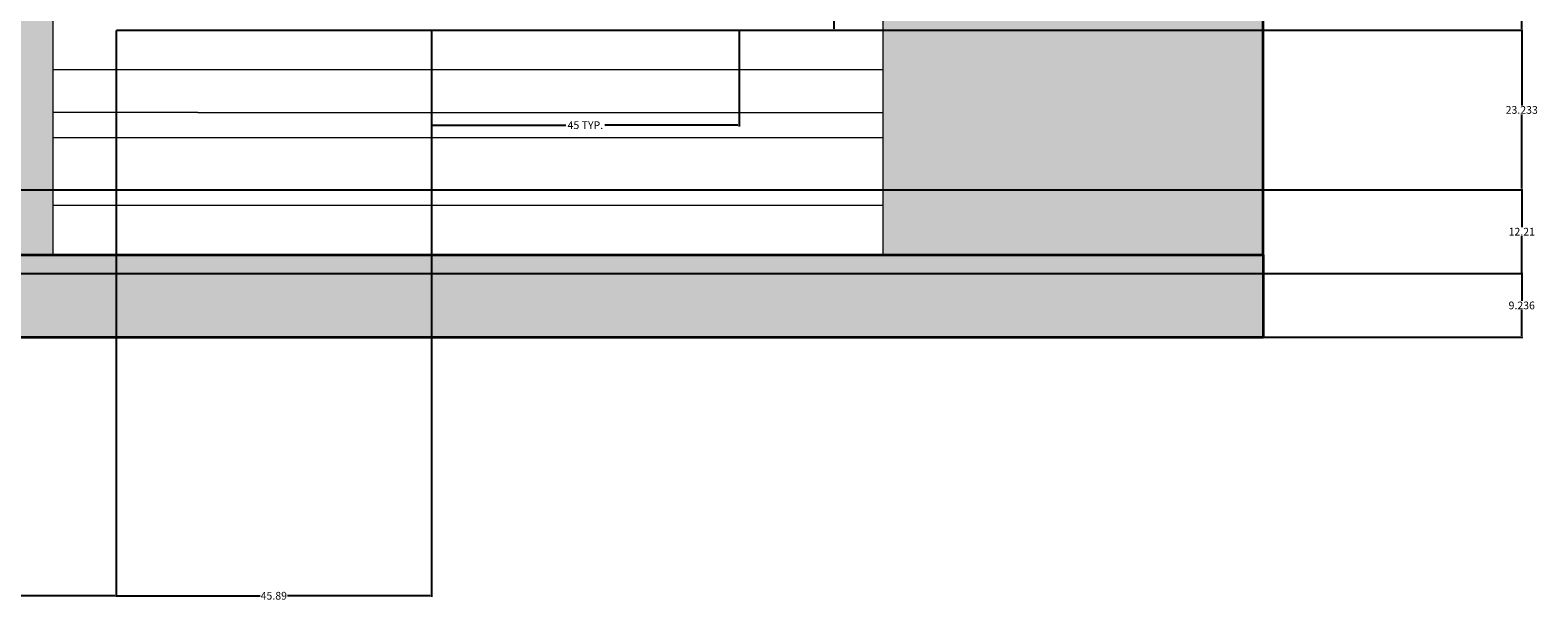
# Model space of a CAD drawing. Units: inches. Extents: x 8 to 634, y 41 to 867.
# Tile 8 of 21: x 415 to 634, y 41 to 124. Entities that reach past the tile are written whole.
import ezdxf

# ---------------------------------------------------------------- set-up
doc = ezdxf.new("R2010")
doc.units = ezdxf.units.IN
doc.header["$MEASUREMENT"] = 0
for name, color, linetype, lineweight in [('A-ANNO-DIMS', 2, 'Continuous', 18), ('A-FLOR', 7, 'Continuous', 35), ('A-FLOR-PATT', 8, 'Continuous', 9), ('A-WALL', 7, 'Continuous', 35), ('A-WALL-PANL', 7, 'Continuous', 18), ('A-WALL-PATT', 8, 'Continuous', 9)]:
    doc.layers.add(name, color=color, linetype=linetype, lineweight=lineweight)
doc.styles.get("Standard").update_dxf_attribs({"font": 'arial.ttf'})
doc.dimstyles.get("Standard").update_dxf_attribs({"dimtxt": 1.125, "dimasz": 0.18, "dimexe": 0.18, "dimexo": 0.0625, "dimgap": 0.09, "dimtad": 0, "dimtih": 1, "dimtoh": 1, "dimdec": 4, "dimzin": 0, "dimdsep": 46, "dimlunit": 4, "dimtxsty": 'Standard', "dimcen": 0.09, "dimadec": 0, "dimazin": 0, "dimtfac": 1, "dimtdec": 4, "dimtofl": 0, "dimtmove": 0, "dimatfit": 3, "dimfxl": 1, "dimtolj": 1, "dimtzin": 0, "dimarcsym": 0})

# ---------------------------------------------------------------- blocks, each defined once
blk = doc.blocks.new('*D9')
at = {"layer": 'A-ANNO-DIMS', "color": 0, "lineweight": -2, "transparency": 16777216}
for p, q in [((518.18, 216.5), (532.13, 216.5)), ((531.95, 216.32), (531.95, 171.04)), ((531.95, 124.41), (531.95, 169.69)), ((518.18, 124.23), (532.13, 124.23))]:
    blk.add_line(p, q, dxfattribs=at)
at = {"layer": 'A-ANNO-DIMS', "color": 0, "transparency": 16777216}
for points in [[(531.92, 216.32), (531.98, 216.32), (531.95, 216.5)], [(531.92, 124.41), (531.98, 124.41), (531.95, 124.23)]]:
    blk.add_solid(points, dxfattribs=at)
at = {"layer": 'Defpoints', "color": 0, "transparency": 16777216}
for p in [(518.11, 216.5), (531.95, 216.5), (518.11, 124.23)]:
    blk.add_point(p, dxfattribs=at)
at = {"layer": 'A-ANNO-DIMS', "color": 0, "transparency": 16777216, "insert": (531.95, 170.36), "char_height": 1.125, "attachment_point": 5}
blk.add_mtext('\\A1;TRANSOM WINDOW 92 TYP.', dxfattribs=at)
blk = doc.blocks.new('*D10')
at = {"layer": 'A-ANNO-DIMS', "color": 0, "lineweight": -2, "transparency": 16777216}
for p, q in [((473.33, 124.17), (473.33, 110.22)), ((518.11, 124.17), (518.11, 110.22)), ((473.51, 110.4), (492.87, 110.4)), ((517.93, 110.4), (498.57, 110.4))]:
    blk.add_line(p, q, dxfattribs=at)
at = {"layer": 'A-ANNO-DIMS', "color": 0, "transparency": 16777216}
for points in [[(473.51, 110.43), (473.51, 110.37), (473.33, 110.4)], [(517.93, 110.43), (517.93, 110.37), (518.11, 110.4)]]:
    blk.add_solid(points, dxfattribs=at)
at = {"layer": 'Defpoints', "color": 0, "transparency": 16777216}
for p in [(473.33, 124.23), (518.11, 124.23), (518.11, 110.4)]:
    blk.add_point(p, dxfattribs=at)
at = {"layer": 'A-ANNO-DIMS', "color": 0, "transparency": 16777216, "insert": (495.72, 110.4), "char_height": 1.125, "attachment_point": 5}
blk.add_mtext('\\A1;45 TYP.', dxfattribs=at)
blk = doc.blocks.new('*D32')
at = {"layer": 'A-ANNO-DIMS', "color": 0, "lineweight": -2, "transparency": 16777216}
for p, q in [((427.44, 124.17), (427.44, 41.73)), ((353.46, 100.94), (353.46, 41.73)), ((353.64, 41.91), (388.46, 41.91)), ((427.26, 41.91), (392.43, 41.91))]:
    blk.add_line(p, q, dxfattribs=at)
at = {"layer": 'A-ANNO-DIMS', "color": 0, "transparency": 16777216}
for points in [[(353.64, 41.94), (353.64, 41.88), (353.46, 41.91)], [(427.26, 41.94), (427.26, 41.88), (427.44, 41.91)]]:
    blk.add_solid(points, dxfattribs=at)
at = {"layer": 'Defpoints', "color": 0, "transparency": 16777216}
for p in [(427.44, 124.23), (353.46, 101), (427.44, 41.91)]:
    blk.add_point(p, dxfattribs=at)
at = {"layer": 'A-ANNO-DIMS', "color": 0, "transparency": 16777216, "insert": (390.45, 41.91), "char_height": 1.125, "attachment_point": 5}
blk.add_mtext('\\A1;73.98', dxfattribs=at)
blk = doc.blocks.new('*D33')
at = {"layer": 'A-ANNO-DIMS', "color": 0, "lineweight": -2, "transparency": 16777216}
for p, q in [((427.44, 124.17), (427.44, 41.73)), ((473.33, 124.17), (473.33, 41.73)), ((427.62, 41.91), (448.37, 41.91)), ((473.15, 41.91), (452.39, 41.91))]:
    blk.add_line(p, q, dxfattribs=at)
at = {"layer": 'A-ANNO-DIMS', "color": 0, "transparency": 16777216}
for points in [[(427.62, 41.94), (427.62, 41.88), (427.44, 41.91)], [(473.15, 41.94), (473.15, 41.88), (473.33, 41.91)]]:
    blk.add_solid(points, dxfattribs=at)
at = {"layer": 'Defpoints', "color": 0, "transparency": 16777216}
for p in [(427.44, 124.23), (473.33, 124.23), (473.33, 41.91)]:
    blk.add_point(p, dxfattribs=at)
at = {"layer": 'A-ANNO-DIMS', "color": 0, "transparency": 16777216, "insert": (450.38, 41.91), "char_height": 1.125, "attachment_point": 5}
blk.add_mtext('\\A1;45.89', dxfattribs=at)
blk = doc.blocks.new('*D36')
at = {"layer": 'A-ANNO-DIMS', "color": 0, "lineweight": -2, "transparency": 16777216}
for p, q in [((269.06, 88.79), (632.18, 88.79)), ((632, 88.61), (632, 84.84)), ((632, 79.74), (632, 83.51)), ((594.41, 79.56), (632.18, 79.56))]:
    blk.add_line(p, q, dxfattribs=at)
at = {"layer": 'A-ANNO-DIMS', "color": 0, "transparency": 16777216}
for points in [[(631.97, 88.61), (632.03, 88.61), (632, 88.79)], [(631.97, 79.74), (632.03, 79.74), (632, 79.56)]]:
    blk.add_solid(points, dxfattribs=at)
at = {"layer": 'Defpoints', "color": 0, "transparency": 16777216}
for p in [(269, 88.79), (632, 88.79), (594.35, 79.56)]:
    blk.add_point(p, dxfattribs=at)
at = {"layer": 'A-ANNO-DIMS', "color": 0, "transparency": 16777216, "insert": (632, 84.17), "char_height": 1.125, "attachment_point": 5}
blk.add_mtext('\\A1;9.236', dxfattribs=at)
blk = doc.blocks.new('*D37')
at = {"layer": 'A-ANNO-DIMS', "color": 0, "lineweight": -2, "transparency": 16777216}
for p, q in [((353.52, 101), (632.18, 101)), ((632, 100.82), (632, 95.55)), ((632, 88.97), (632, 94.24)), ((269.06, 88.79), (632.18, 88.79))]:
    blk.add_line(p, q, dxfattribs=at)
at = {"layer": 'A-ANNO-DIMS', "color": 0, "transparency": 16777216}
for points in [[(631.97, 100.82), (632.03, 100.82), (632, 101)], [(631.97, 88.97), (632.03, 88.97), (632, 88.79)]]:
    blk.add_solid(points, dxfattribs=at)
at = {"layer": 'Defpoints', "color": 0, "transparency": 16777216}
for p in [(353.46, 101), (632, 101), (269, 88.79)]:
    blk.add_point(p, dxfattribs=at)
at = {"layer": 'A-ANNO-DIMS', "color": 0, "transparency": 16777216, "insert": (632, 94.9), "char_height": 1.125, "attachment_point": 5}
blk.add_mtext('\\A1;12.21', dxfattribs=at)
blk = doc.blocks.new('*D38')
at = {"layer": 'A-ANNO-DIMS', "color": 0, "lineweight": -2, "transparency": 16777216}
for p, q in [((427.5, 124.23), (632.18, 124.23)), ((632, 124.05), (632, 113.28)), ((632, 101.18), (632, 111.95)), ((353.52, 101), (632.18, 101))]:
    blk.add_line(p, q, dxfattribs=at)
at = {"layer": 'A-ANNO-DIMS', "color": 0, "transparency": 16777216}
for points in [[(631.97, 124.05), (632.03, 124.05), (632, 124.23)], [(631.97, 101.18), (632.03, 101.18), (632, 101)]]:
    blk.add_solid(points, dxfattribs=at)
at = {"layer": 'Defpoints', "color": 0, "transparency": 16777216}
for p in [(427.44, 124.23), (632, 124.23), (353.46, 101)]:
    blk.add_point(p, dxfattribs=at)
at = {"layer": 'A-ANNO-DIMS', "color": 0, "transparency": 16777216, "insert": (632, 112.62), "char_height": 1.125, "attachment_point": 5}
blk.add_mtext('\\A1;23.233', dxfattribs=at)
blk = doc.blocks.new('*D39')
at = {"layer": 'A-ANNO-DIMS', "color": 0, "lineweight": -2, "transparency": 16777216}
for p, q in [((427.5, 288.17), (632.18, 288.17)), ((632, 287.99), (632, 206.86)), ((632, 124.41), (632, 205.54)), ((427.5, 124.23), (632.18, 124.23))]:
    blk.add_line(p, q, dxfattribs=at)
at = {"layer": 'A-ANNO-DIMS', "color": 0, "transparency": 16777216}
for points in [[(631.97, 287.99), (632.03, 287.99), (632, 288.17)], [(631.97, 124.41), (632.03, 124.41), (632, 124.23)]]:
    blk.add_solid(points, dxfattribs=at)
at = {"layer": 'Defpoints', "color": 0, "transparency": 16777216}
for p in [(427.44, 288.17), (632, 288.17), (427.44, 124.23)]:
    blk.add_point(p, dxfattribs=at)
at = {"layer": 'A-ANNO-DIMS', "color": 0, "transparency": 16777216, "insert": (632, 206.2), "char_height": 1.125, "attachment_point": 5}
blk.add_mtext('\\A1;163.93', dxfattribs=at)

msp = doc.modelspace()

# ---------------------------------------------------------------- hatches: boundary and pattern name
at = {"layer": 'A-FLOR-PATT', "transparency": 33554687}
h = msp.add_hatch(dxfattribs=at)
h.set_pattern_fill('AR-CONC', color=256, scale=0.76, angle=135)
h.set_pattern_definition([(185, (0, 0), (-3.517334, 4.191795), [0.57, -6.27]), (130, (0, 0), (-3.29664, -4.78794), [0.456, -5.016]), (235.4514, (-0.293, 0.3493), (-6.81397, -0.596145), [0.484425, -5.32868]), (181.1842, (-1.075, -1.075), (-4.845865, 6.62487), [0.855, -9.405]), (231.6356, (-1.479, -0.523), (-10.25781, -0.21204), [0.72664, -7.99302]), (126.1842, (-1.075, -1.075), (-10.25781, -0.21204), [0.684, -7.524]), (156, (-1.3435, -0.2687), (-1.044107, 5.371464), [0.57, -6.27]), (101, (-1.3435, -0.2687), (-5.204544, -2.589385), [0.456, -5.016]), (206.4514, (-1.4305, 0.179), (-6.24865, 2.78208), [0.484425, -5.32868]), (172.5, (0, 0), (-1.8543226, -1.723628), [0, -4.9552, 0, -5.092, 0, -5.035]), (142.5, (0, 0), (-3.533312, -0.705834), [0, -2.9032, 0, -4.8412, 0, -1.919]), (102.5, (1.1984, -1.1984), (-2.747558, 2.989978), [0, -1.9, 0, -5.928, 0, -7.866]), (92.5, (1.7358, -1.7358), (-3.672015, 2.596084), [0, -2.47, 0, -3.9368, 0, -5.586])])
h.paths.add_polyline_path([(594.3501, 91.5417), (360.785, 91.5417), (295.0049, 91.5417), (268.998, 91.5432), (268.998, 88.7912), (63.5448, 88.7912), (63.5448, 91.5555), (47.3401, 91.5555), (47.3401, 79.5555), (349.489, 79.5555), (594.3501, 79.5555)])
at = {"layer": 'A-WALL-PATT', "transparency": 33554687}
h = msp.add_hatch(dxfattribs=at)
h.set_pattern_fill('ANSI31', color=256, scale=79, angle=135)
h.paths.add_polyline_path([(539.0002, 276.166), (499.4677, 276.166), (418.2881, 276.166), (418.2881, 228.4951), (435.5682, 228.4951), (539.0002, 228.4951)])
h.paths.add_polyline_path([(539.0002, 228.4951), (435.5682, 228.4951), (418.2881, 228.4951), (418.2881, 112.2342), (439.3242, 112.2342), (539.0002, 112.2342)])
h.paths.add_polyline_path([(518.1129, 124.2342), (473.3277, 124.2342), (473.3277, 216.4951), (518.1129, 216.4951)], flags=16)
h.paths.add_polyline_path([(451.2116, 124.2342), (427.4368, 124.2342), (427.4368, 216.4951), (451.2116, 216.4951)], flags=16)
h.paths.add_polyline_path([(539.0002, 112.2342), (439.3242, 112.2342), (418.2881, 112.2342), (418.2881, 91.5417), (539.0002, 91.5417)])
h.paths.add_polyline_path([(539.0002, 392.4268), (427.4368, 392.4268), (418.2881, 392.4268), (418.2881, 391.7598), (418.2881, 276.166), (499.4677, 276.166), (539.0002, 276.166)])
h.paths.add_polyline_path([(518.1129, 288.166), (473.3277, 288.166), (473.3277, 380.4268), (518.1129, 380.4268)], flags=16)
h.paths.add_polyline_path([(451.2116, 288.166), (427.4368, 288.166), (427.4368, 380.4268), (451.2116, 380.4268)], flags=16)
h.paths.add_polyline_path([(539.0002, 451.6305), (427.4368, 452.9097), (418.2881, 452.9097), (418.2881, 392.4268), (427.4368, 392.4268), (539.0002, 392.4268)])
h.paths.add_polyline_path([(539.0002, 569.1705), (427.4368, 569.1705), (418.2881, 569.1705), (418.2881, 452.9097), (427.4368, 452.9097), (539.0002, 451.6305)])
h.paths.add_polyline_path([(473.3277, 557.1705), (518.1129, 557.1705), (518.1129, 464.9097), (473.3277, 464.9097)], flags=16)
h.paths.add_polyline_path([(451.2116, 557.1705), (451.2116, 464.9097), (427.4368, 464.9097), (427.4368, 557.1705)], flags=16)
h.paths.add_polyline_path([(539.0002, 619.6298), (418.2881, 619.6298), (418.2881, 569.1705), (427.4368, 569.1705), (539.0002, 569.1705)])
h.paths.add_polyline_path([(556.7072, 774.3342), (556.7072, 776.8929), (299.7961, 776.8929), (299.7961, 697.6655), (322.56, 697.6655), (322.56, 740.5561), (355.7466, 740.5561), (355.7466, 697.6655), (360.785, 697.6655), (370.3877, 697.6655), (370.3877, 740.5561), (439.201, 740.5561), (439.201, 691.978), (449.4498, 691.978), (449.4498, 740.5561), (498.2535, 740.5561), (498.2535, 691.978), (508.5023, 691.978), (508.5023, 740.5561), (536.3204, 740.5561), (536.3204, 691.978), (539.0002, 691.978), (539.0002, 697.6655), (556.7072, 697.6655)])
h = msp.add_hatch(dxfattribs=at)
h.set_pattern_fill('AR-CONC', color=256, scale=3.2)
h.paths.add_polyline_path([(119.7065, 697.6655), (47.3401, 697.6655), (47.3401, 569.1705), (119.7065, 569.1705)])
h.paths.add_polyline_path([(202.1558, 697.6655), (119.7065, 697.6655), (119.7065, 569.1705), (202.1558, 569.1705)])
h.paths.add_polyline_path([(284.6051, 697.6655), (202.1558, 697.6655), (202.1558, 569.1705), (284.6051, 569.1705)])
h.paths.add_polyline_path([(119.7065, 569.1705), (47.3401, 569.1705), (47.3401, 523.5555), (47.3401, 449.7533), (119.7065, 449.7533)])
h.paths.add_polyline_path([(342.6544, 682.1444), (360.785, 697.6655), (284.6051, 697.6655), (284.6051, 569.1705), (342.6544, 569.1705)])
h.paths.add_polyline_path([(342.6544, 569.1705), (284.6051, 569.1705), (284.6051, 449.7533), (342.6544, 449.7533)])
h.paths.add_polyline_path([(418.2881, 691.978), (418.2881, 697.6655), (360.785, 697.6655), (360.785, 569.1705), (418.2881, 569.1705)])
h.paths.add_polyline_path([(418.2881, 569.1705), (360.785, 569.1705), (360.785, 523.5555), (360.785, 449.7533), (418.2881, 449.7533)])
h.paths.add_polyline_path([(594.3501, 697.6655), (539.0002, 697.6655), (539.0002, 691.978), (539.0002, 569.1705), (594.3501, 569.1705)])
h.paths.add_polyline_path([(594.3501, 523.5555), (594.3501, 569.1705), (539.0002, 569.1705), (539.0002, 451.6305), (594.3501, 451.6305)])
h.paths.add_polyline_path([(594.3501, 451.6305), (539.0002, 451.6305), (539.0002, 391.7598), (594.3501, 391.7598)])
h.paths.add_polyline_path([(594.3501, 391.7598), (539.0002, 391.7598), (539.0002, 276.166), (594.3501, 276.166)])
h.paths.add_polyline_path([(418.2881, 449.7533), (360.785, 449.7533), (360.785, 391.7598), (418.2881, 391.7598)])
h.paths.add_polyline_path([(342.6544, 449.7533), (284.6051, 449.7533), (284.6051, 391.7598), (342.6544, 391.7598)])
h.paths.add_polyline_path([(342.6544, 391.7598), (284.6051, 391.7598), (284.6051, 272.3426), (342.6544, 272.3426)])
h.paths.add_polyline_path([(418.2881, 391.7598), (360.785, 391.7598), (360.785, 272.3426), (418.2881, 272.3426)])
h.paths.add_polyline_path([(418.2881, 272.3426), (360.785, 272.3426), (360.785, 235.5555), (418.2881, 235.5555)])
h.paths.add_polyline_path([(342.6544, 272.3426), (284.6051, 272.3426), (284.6051, 235.5555), (295.0049, 235.5555), (342.6544, 235.5555)])
h.paths.add_polyline_path([(594.3501, 276.166), (539.0002, 276.166), (539.0002, 228.4951), (594.3501, 228.4951)])
h.paths.add_polyline_path([(594.3501, 228.4951), (539.0002, 228.4951), (539.0002, 91.5417), (594.3501, 91.5417)])
h.paths.add_polyline_path([(418.2881, 235.5555), (360.785, 235.5555), (360.785, 91.5417), (418.2881, 91.5417)])
h.paths.add_polyline_path([(284.6051, 272.3426), (119.7065, 272.3426), (119.7065, 235.5555), (284.6051, 235.5555)])
h.paths.add_polyline_path([(119.7065, 272.3426), (47.3401, 272.3426), (47.3401, 235.5555), (47.3401, 91.5555), (63.5448, 91.5555), (63.5448, 227.8036), (268.998, 227.8036), (268.998, 91.5555), (295.0049, 91.5555), (295.0049, 222.583), (271.9787, 222.583), (271.9787, 229.0481), (62.4019, 229.0481), (62.4019, 222.583), (61.1827, 222.583), (61.1827, 235.5555), (119.7065, 235.5555)])
h.paths.add_polyline_path([(119.7065, 391.7598), (47.3401, 391.7598), (47.3401, 379.5555), (47.3401, 272.3426), (119.7065, 272.3426)])
h.paths.add_polyline_path([(119.7065, 449.7533), (47.3401, 449.7533), (47.3401, 391.7598), (119.7065, 391.7598)])
h.paths.add_polyline_path([(202.1558, 449.7533), (119.7065, 449.7533), (119.7065, 391.7598), (202.1558, 391.7598)])
h.paths.add_polyline_path([(284.6051, 449.7533), (202.1558, 449.7533), (202.1558, 391.7598), (284.6051, 391.7598)])

# ---------------------------------------------------------------- linework, layer by layer
at = {"layer": 'A-FLOR'}
for p, q in [((360.785, 91.5417), (594.3501, 91.5417)), ((594.3501, 91.5417), (594.3501, 79.5555)), ((349.489, 79.5555), (594.3501, 79.5555))]:
    msp.add_line(p, q, dxfattribs=at)
at = {"layer": 'A-WALL'}
msp.add_line((594.3501, 91.5417), (594.3501, 523.5555), dxfattribs=at)
at = {"layer": 'A-WALL-PANL'}
for q in [(418.2881, 112.2342), (539.0002, 112.2342)]:
    msp.add_line((439.3242, 112.2342), q, dxfattribs=at)
msp.add_lwpolyline([(539.0002, 691.978), (539.0002, 91.5417), (418.2881, 91.5417), (418.2881, 691.978)], dxfattribs=at)

# ---------------------------------------------------------------- dimensions: what is measured, and where the dimension line sits
at = {"layer": 'A-ANNO-DIMS'}
for base, p1, p2, override, picture, middle in [((632.0001, 288.166), (427.4368, 124.2342), (427.4368, 288.166), {"dimdec": 2, "dimlfac": 1, "dimrnd": 0, "dimzin": 0, "dimdsep": 46, "dimlunit": 2}, '*D39', (632.0001, 206.2001)), ((632.0001, 124.2342), (353.4573, 101.0012), (427.4368, 124.2342), {"dimdec": 3, "dimlfac": 1, "dimrnd": 0, "dimzin": 0, "dimdsep": 46, "dimlunit": 2}, '*D38', (632.0001, 112.6177)), ((632.0001, 101.0012), (268.998, 88.7912), (353.4573, 101.0012), {"dimdec": 2, "dimlfac": 1, "dimrnd": 0, "dimzin": 0, "dimdsep": 46, "dimlunit": 2}, '*D37', (632.0001, 94.8962)), ((632.0001, 88.7912), (594.3501, 79.5555), (268.998, 88.7912), {"dimdec": 3, "dimlfac": 1, "dimrnd": 0, "dimzin": 0, "dimdsep": 46, "dimlunit": 2}, '*D36', (632.0001, 84.1734))]:
    dim = msp.add_linear_dim(base=base, p1=p1, p2=p2, angle=90, dimstyle='Standard', override=override, dxfattribs=at)
    dim.commit()
    dim.dimension.update_dxf_attribs({"geometry": picture, "text_midpoint": middle})
dim = msp.add_linear_dim(base=(531.952, 216.4951), p1=(518.1129, 124.2342), p2=(518.1129, 216.4951), angle=90, text='TRANSOM WINDOW <> TYP.', dimstyle='Standard', override={"dimdec": 0, "dimlfac": 1, "dimrnd": 0, "dimzin": 0, "dimdsep": 46, "dimlunit": 2}, dxfattribs=at)
dim.commit()
dim.dimension.update_dxf_attribs({"geometry": '*D9', "text_midpoint": (531.952, 170.3647)})
for base, p1, p2, picture, middle in [((427.4368, 41.9055), (353.4573, 101.0012), (427.4368, 124.2342), '*D32', (390.447, 41.9055)), ((473.3277, 41.9055), (427.4368, 124.2342), (473.3277, 124.2342), '*D33', (450.3823, 41.9055))]:
    dim = msp.add_linear_dim(base=base, p1=p1, p2=p2, dimstyle='Standard', override={"dimdec": 2, "dimlfac": 1, "dimrnd": 0, "dimzin": 0, "dimdsep": 46, "dimlunit": 2}, dxfattribs=at)
    dim.commit()
    dim.dimension.update_dxf_attribs({"geometry": picture, "text_midpoint": middle})
dim = msp.add_linear_dim(base=(518.1129, 110.3951), p1=(473.3277, 124.2342), p2=(518.1129, 124.2342), text='<> TYP.', dimstyle='Standard', override={"dimdec": 0, "dimlfac": 1, "dimrnd": 0, "dimzin": 0, "dimdsep": 46, "dimlunit": 2}, dxfattribs=at)
dim.commit()
dim.dimension.update_dxf_attribs({"geometry": '*D10', "text_midpoint": (495.7203, 110.3951)})

doc.saveas('drawing.dxf')
